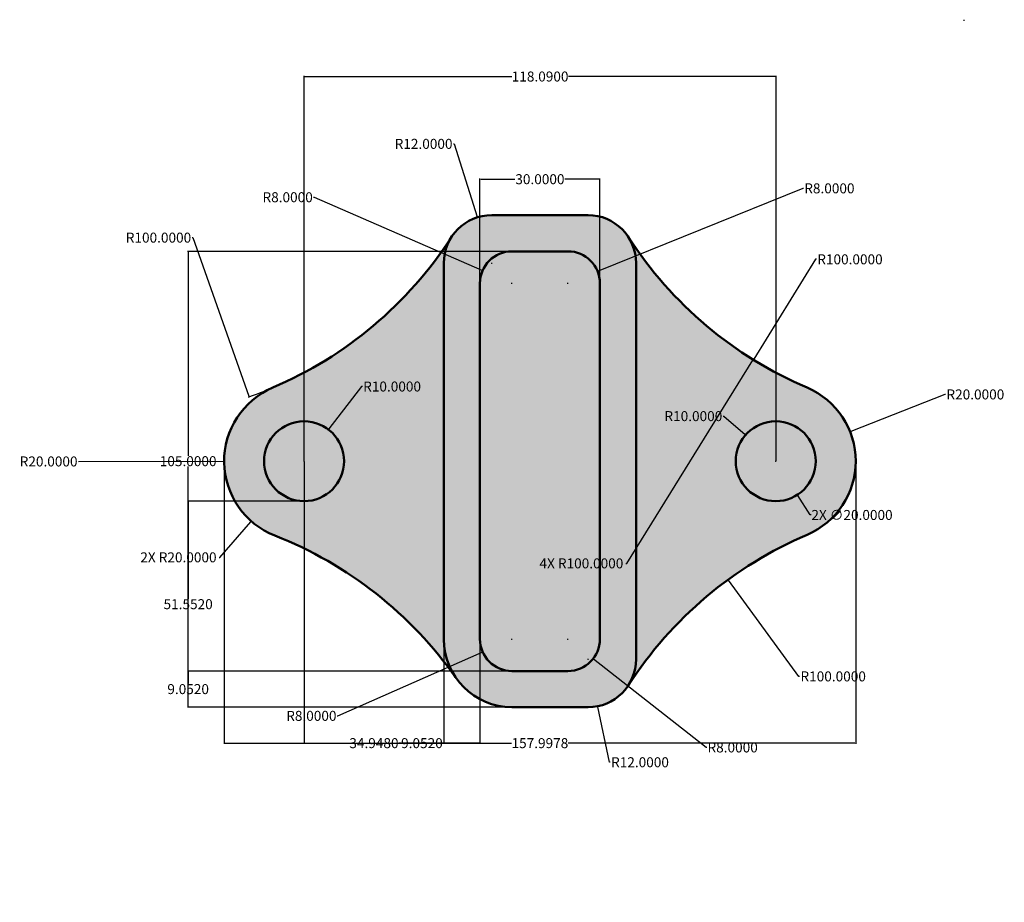
# Model space of a CAD drawing. Units: inches. Extents: x 2167893 to 2168140, y 2398931 to 2399152.
import ezdxf

# ---------------------------------------------------------------- set-up
doc = ezdxf.new("R2010")
doc.units = ezdxf.units.IN
doc.header["$MEASUREMENT"] = 0
for name, color, linetype, lineweight in [('M-DIMS', 2, 'Continuous', 25), ('M-HATC', 8, 'Continuous', 18), ('M-OUTL', 7, 'Continuous', 50)]:
    doc.layers.add(name, color=color, linetype=linetype, lineweight=lineweight)
doc.styles.get("Standard").update_dxf_attribs({"font": 'arial.ttf'})
doc.dimstyles.get("Standard").update_dxf_attribs({"dimtxt": 2.5, "dimasz": 0.18, "dimexe": 0.18, "dimexo": 0.0625, "dimgap": 0.09, "dimtad": 0, "dimtih": 1, "dimtoh": 1, "dimdec": 4, "dimzin": 0, "dimdsep": 46, "dimtxsty": 'Standard', "dimcen": 0.09, "dimadec": 0, "dimazin": 0, "dimtfac": 1, "dimtdec": 4, "dimtofl": 0, "dimtmove": 0, "dimatfit": 3, "dimfxl": 1, "dimtolj": 1, "dimtzin": 0, "dimarcsym": 0})

# ---------------------------------------------------------------- blocks, each defined once
blk = doc.blocks.new('*D1')
at = {"layer": 'Defpoints', "color": 0, "transparency": 16777216}
for p in [(2168070.68, 2399011.55), (2168129.7, 2398930.83)]:
    blk.add_point(p, dxfattribs=at)
at = {"layer": 'M-DIMS', "color": 0, "lineweight": -2, "transparency": 16777216}
for p, q in [((2168088.38, 2398987.35), (2168070.79, 2399011.41)), ((2168088.56, 2398987.35), (2168088.38, 2398987.35))]:
    blk.add_line(p, q, dxfattribs=at)
at = {"layer": 'M-DIMS', "color": 0, "transparency": 16777216}
blk.add_solid([(2168070.81, 2399011.42), (2168070.76, 2399011.39), (2168070.68, 2399011.55)], dxfattribs=at)
at = {"layer": 'M-DIMS', "color": 0, "transparency": 16777216, "insert": (2168096.97, 2398987.35), "char_height": 2.5, "attachment_point": 5}
blk.add_mtext('\\A1;R100.0000', dxfattribs=at)
blk = doc.blocks.new('*D2')
at = {"layer": 'Defpoints', "color": 0, "transparency": 16777216}
for p in [(2168075.05, 2399047.75), (2168082.6, 2399041.2)]:
    blk.add_point(p, dxfattribs=at)
at = {"layer": 'M-DIMS', "color": 0, "lineweight": -2, "transparency": 16777216}
for p, q in [((2168069.43, 2399052.47), (2168069.61, 2399052.47)), ((2168069.61, 2399052.47), (2168074.91, 2399047.87)), ((2168082.51, 2399041.2), (2168082.69, 2399041.2)), ((2168082.6, 2399041.11), (2168082.6, 2399041.29))]:
    blk.add_line(p, q, dxfattribs=at)
at = {"layer": 'M-DIMS', "color": 0, "transparency": 16777216}
blk.add_solid([(2168074.93, 2399047.89), (2168074.9, 2399047.85), (2168075.05, 2399047.75)], dxfattribs=at)
at = {"layer": 'M-DIMS', "color": 0, "transparency": 16777216, "insert": (2168061.99, 2399052.47), "char_height": 2.5, "attachment_point": 5}
blk.add_mtext('\\A1;R10.0000', dxfattribs=at)
blk = doc.blocks.new('*D3')
at = {"layer": 'Defpoints', "color": 0, "transparency": 16777216}
for p in [(2168101.21, 2399048.54), (2168082.6, 2399041.2)]:
    blk.add_point(p, dxfattribs=at)
at = {"layer": 'M-DIMS', "color": 0, "lineweight": -2, "transparency": 16777216}
for p, q in [((2168124.92, 2399057.9), (2168101.37, 2399048.61)), ((2168125.1, 2399057.9), (2168124.92, 2399057.9)), ((2168082.51, 2399041.2), (2168082.69, 2399041.2)), ((2168082.6, 2399041.11), (2168082.6, 2399041.29))]:
    blk.add_line(p, q, dxfattribs=at)
at = {"layer": 'M-DIMS', "color": 0, "transparency": 16777216}
blk.add_solid([(2168101.36, 2399048.63), (2168101.38, 2399048.58), (2168101.21, 2399048.54)], dxfattribs=at)
at = {"layer": 'M-DIMS', "color": 0, "transparency": 16777216, "insert": (2168132.54, 2399057.9), "char_height": 2.5, "attachment_point": 5}
blk.add_mtext('\\A1;R20.0000', dxfattribs=at)
blk = doc.blocks.new('*D4')
at = {"layer": 'Defpoints', "color": 0, "transparency": 16777216}
for p in [(2168129.7, 2399151.57), (2168077, 2399066.58)]:
    blk.add_point(p, dxfattribs=at)
at = {"layer": 'M-DIMS', "color": 0, "lineweight": -2, "transparency": 16777216}
for p, q in [((2168092.58, 2399091.7), (2168077.1, 2399066.74)), ((2168092.76, 2399091.7), (2168092.58, 2399091.7))]:
    blk.add_line(p, q, dxfattribs=at)
at = {"layer": 'M-DIMS', "color": 0, "transparency": 16777216}
blk.add_solid([(2168077.07, 2399066.75), (2168077.12, 2399066.72), (2168077, 2399066.58)], dxfattribs=at)
at = {"layer": 'M-DIMS', "color": 0, "transparency": 16777216, "insert": (2168101.17, 2399091.7), "char_height": 2.5, "attachment_point": 5}
blk.add_mtext('\\A1;R100.0000', dxfattribs=at)
blk = doc.blocks.new('*D5')
at = {"layer": 'Defpoints', "color": 0, "transparency": 16777216}
for p in [(2168030.6, 2398996.7), (2168036.9, 2398991.76)]:
    blk.add_point(p, dxfattribs=at)
at = {"layer": 'M-DIMS', "color": 0, "lineweight": -2, "transparency": 16777216}
for p, q in [((2168030.51, 2398996.7), (2168030.69, 2398996.7)), ((2168030.6, 2398996.61), (2168030.6, 2398996.79)), ((2168065.17, 2398969.58), (2168037.04, 2398991.65)), ((2168065.35, 2398969.58), (2168065.17, 2398969.58))]:
    blk.add_line(p, q, dxfattribs=at)
at = {"layer": 'M-DIMS', "color": 0, "transparency": 16777216}
blk.add_solid([(2168037.06, 2398991.67), (2168037.02, 2398991.63), (2168036.9, 2398991.76)], dxfattribs=at)
at = {"layer": 'M-DIMS', "color": 0, "transparency": 16777216, "insert": (2168071.82, 2398969.58), "char_height": 2.5, "attachment_point": 5}
blk.add_mtext('\\A1;R8.0000', dxfattribs=at)
blk = doc.blocks.new('*D6')
at = {"layer": 'Defpoints', "color": 0, "transparency": 16777216}
for p in [(2168016.6, 2398996.7), (2168009.28, 2398993.47)]:
    blk.add_point(p, dxfattribs=at)
at = {"layer": 'M-DIMS', "color": 0, "lineweight": -2, "transparency": 16777216}
for p, q in [((2168016.51, 2398996.7), (2168016.69, 2398996.7)), ((2168016.6, 2398996.61), (2168016.6, 2398996.79)), ((2167973.07, 2398977.48), (2168009.12, 2398993.39)), ((2167972.89, 2398977.48), (2167973.07, 2398977.48))]:
    blk.add_line(p, q, dxfattribs=at)
at = {"layer": 'M-DIMS', "color": 0, "transparency": 16777216}
blk.add_solid([(2168009.11, 2398993.42), (2168009.13, 2398993.37), (2168009.28, 2398993.47)], dxfattribs=at)
at = {"layer": 'M-DIMS', "color": 0, "transparency": 16777216, "insert": (2167966.42, 2398977.48), "char_height": 2.5, "attachment_point": 5}
blk.add_mtext('\\A1;R8.0000', dxfattribs=at)
blk = doc.blocks.new('*D7')
at = {"layer": 'Defpoints', "color": 0, "transparency": 16777216}
for p in [(2168038.02, 2399088.7), (2168030.6, 2399085.7)]:
    blk.add_point(p, dxfattribs=at)
at = {"layer": 'M-DIMS', "color": 0, "lineweight": -2, "transparency": 16777216}
for p, q in [((2168089.37, 2399109.46), (2168038.19, 2399088.76)), ((2168089.55, 2399109.46), (2168089.37, 2399109.46)), ((2168030.51, 2399085.7), (2168030.69, 2399085.7)), ((2168030.6, 2399085.61), (2168030.6, 2399085.79))]:
    blk.add_line(p, q, dxfattribs=at)
at = {"layer": 'M-DIMS', "color": 0, "transparency": 16777216}
blk.add_solid([(2168038.17, 2399088.79), (2168038.2, 2399088.74), (2168038.02, 2399088.7)], dxfattribs=at)
at = {"layer": 'M-DIMS', "color": 0, "transparency": 16777216, "insert": (2168096.02, 2399109.46), "char_height": 2.5, "attachment_point": 5}
blk.add_mtext('\\A1;R8.0000', dxfattribs=at)
blk = doc.blocks.new('*D8')
at = {"layer": 'Defpoints', "color": 0, "transparency": 16777216}
for p in [(2168009.27, 2399088.89), (2168016.6, 2399085.7)]:
    blk.add_point(p, dxfattribs=at)
at = {"layer": 'M-DIMS', "color": 0, "lineweight": -2, "transparency": 16777216}
for p, q in [((2167966.97, 2399107.24), (2167967.15, 2399107.24)), ((2167967.15, 2399107.24), (2168009.1, 2399088.96)), ((2168016.51, 2399085.7), (2168016.69, 2399085.7)), ((2168016.6, 2399085.61), (2168016.6, 2399085.79))]:
    blk.add_line(p, q, dxfattribs=at)
at = {"layer": 'M-DIMS', "color": 0, "transparency": 16777216}
blk.add_solid([(2168009.11, 2399088.99), (2168009.09, 2399088.94), (2168009.27, 2399088.89)], dxfattribs=at)
at = {"layer": 'M-DIMS', "color": 0, "transparency": 16777216, "insert": (2167960.49, 2399107.24), "char_height": 2.5, "attachment_point": 5}
blk.add_mtext('\\A1;R8.0000', dxfattribs=at)
blk = doc.blocks.new('*D9')
at = {"layer": 'Defpoints', "color": 0, "transparency": 16777216}
for p in [(2167917.5, 2399151.57), (2167950.88, 2399057.3)]:
    blk.add_point(p, dxfattribs=at)
at = {"layer": 'M-DIMS', "color": 0, "lineweight": -2, "transparency": 16777216}
for p, q in [((2167936.6, 2399097.13), (2167936.78, 2399097.13)), ((2167936.78, 2399097.13), (2167950.82, 2399057.47))]:
    blk.add_line(p, q, dxfattribs=at)
blk.add_arc((2167917.5, 2399151.57), 100, 289.3936, 293.0748, dxfattribs=at)
at = {"layer": 'M-DIMS', "color": 0, "transparency": 16777216}
blk.add_solid([(2167950.84, 2399057.48), (2167950.79, 2399057.46), (2167950.88, 2399057.3)], dxfattribs=at)
at = {"layer": 'M-DIMS', "color": 0, "transparency": 16777216, "insert": (2167928.18, 2399097.13), "char_height": 2.5, "attachment_point": 5}
blk.add_mtext('\\A1;R100.0000', dxfattribs=at)
blk = doc.blocks.new('*D10')
at = {"layer": 'Defpoints', "color": 0, "transparency": 16777216}
for p in [(2167970.71, 2399049.12), (2167964.6, 2399041.2)]:
    blk.add_point(p, dxfattribs=at)
at = {"layer": 'M-DIMS', "color": 0, "lineweight": -2, "transparency": 16777216}
for p, q in [((2167979, 2399059.88), (2167970.82, 2399049.26)), ((2167979.18, 2399059.88), (2167979, 2399059.88)), ((2167964.51, 2399041.2), (2167964.69, 2399041.2)), ((2167964.6, 2399041.11), (2167964.6, 2399041.29))]:
    blk.add_line(p, q, dxfattribs=at)
at = {"layer": 'M-DIMS', "color": 0, "transparency": 16777216}
blk.add_solid([(2167970.79, 2399049.28), (2167970.84, 2399049.24), (2167970.71, 2399049.12)], dxfattribs=at)
at = {"layer": 'M-DIMS', "color": 0, "transparency": 16777216, "insert": (2167986.62, 2399059.88), "char_height": 2.5, "attachment_point": 5}
blk.add_mtext('\\A1;R10.0000', dxfattribs=at)
blk = doc.blocks.new('*D11')
at = {"layer": 'Defpoints', "color": 0, "transparency": 16777216}
for p in [(2167944.6, 2399041.17), (2167964.6, 2399041.2)]:
    blk.add_point(p, dxfattribs=at)
at = {"layer": 'M-DIMS', "color": 0, "lineweight": -2, "transparency": 16777216}
for p, q in [((2167908.13, 2399041.13), (2167944.42, 2399041.17)), ((2167964.51, 2399041.2), (2167964.69, 2399041.2)), ((2167964.6, 2399041.11), (2167964.6, 2399041.29))]:
    blk.add_line(p, q, dxfattribs=at)
at = {"layer": 'M-DIMS', "color": 0, "transparency": 16777216}
blk.add_solid([(2167944.42, 2399041.2), (2167944.42, 2399041.14), (2167944.6, 2399041.17)], dxfattribs=at)
at = {"layer": 'M-DIMS', "color": 0, "transparency": 16777216, "insert": (2167900.69, 2399041.13), "char_height": 2.5, "attachment_point": 5}
blk.add_mtext('\\A1;R20.0000', dxfattribs=at)
blk = doc.blocks.new('*D12')
at = {"layer": 'Defpoints', "color": 0, "transparency": 16777216}
for p in [(2168007.94, 2399102.19), (2168011.55, 2399090.75)]:
    blk.add_point(p, dxfattribs=at)
at = {"layer": 'M-DIMS', "color": 0, "lineweight": -2, "transparency": 16777216}
for p, q in [((2168001.95, 2399120.59), (2168002.13, 2399120.59)), ((2168002.13, 2399120.59), (2168007.88, 2399102.36)), ((2168011.46, 2399090.75), (2168011.64, 2399090.75)), ((2168011.55, 2399090.66), (2168011.55, 2399090.84))]:
    blk.add_line(p, q, dxfattribs=at)
at = {"layer": 'M-DIMS', "color": 0, "transparency": 16777216}
blk.add_solid([(2168007.91, 2399102.37), (2168007.85, 2399102.36), (2168007.94, 2399102.19)], dxfattribs=at)
at = {"layer": 'M-DIMS', "color": 0, "transparency": 16777216, "insert": (2167994.5, 2399120.59), "char_height": 2.5, "attachment_point": 5}
blk.add_mtext('\\A1;R12.0000', dxfattribs=at)
blk = doc.blocks.new('*D13')
at = {"layer": 'Defpoints', "color": 0, "transparency": 16777216}
for p in [(2168035.65, 2398991.65), (2168038.1, 2398979.9)]:
    blk.add_point(p, dxfattribs=at)
at = {"layer": 'M-DIMS', "color": 0, "lineweight": -2, "transparency": 16777216}
for p, q in [((2168035.56, 2398991.65), (2168035.74, 2398991.65)), ((2168035.65, 2398991.56), (2168035.65, 2398991.74)), ((2168041.01, 2398965.87), (2168038.13, 2398979.72)), ((2168041.19, 2398965.87), (2168041.01, 2398965.87))]:
    blk.add_line(p, q, dxfattribs=at)
at = {"layer": 'M-DIMS', "color": 0, "transparency": 16777216}
blk.add_solid([(2168038.16, 2398979.73), (2168038.1, 2398979.71), (2168038.1, 2398979.9)], dxfattribs=at)
at = {"layer": 'M-DIMS', "color": 0, "transparency": 16777216, "insert": (2168048.64, 2398965.87), "char_height": 2.5, "attachment_point": 5}
blk.add_mtext('\\A1;R12.0000', dxfattribs=at)
blk = doc.blocks.new('*D14')
at = {"layer": 'Defpoints', "color": 0, "transparency": 16777216}
for p in [(2167964.6, 2399137.44), (2167964.6, 2399041.29), (2168082.69, 2399041.2)]:
    blk.add_point(p, dxfattribs=at)
at = {"layer": 'M-DIMS', "color": 0, "lineweight": -2, "transparency": 16777216}
for p, q in [((2167964.6, 2399041.35), (2167964.6, 2399137.62)), ((2167964.78, 2399137.44), (2168016.55, 2399137.44)), ((2168082.51, 2399137.44), (2168030.75, 2399137.44)), ((2168082.69, 2399041.26), (2168082.69, 2399137.62))]:
    blk.add_line(p, q, dxfattribs=at)
at = {"layer": 'M-DIMS', "color": 0, "transparency": 16777216}
for points in [[(2167964.78, 2399137.47), (2167964.78, 2399137.41), (2167964.6, 2399137.44)], [(2168082.51, 2399137.47), (2168082.51, 2399137.41), (2168082.69, 2399137.44)]]:
    blk.add_solid(points, dxfattribs=at)
at = {"layer": 'M-DIMS', "color": 0, "transparency": 16777216, "insert": (2168023.65, 2399137.44), "char_height": 2.5, "attachment_point": 5}
blk.add_mtext('\\A1;118.0900', dxfattribs=at)
blk = doc.blocks.new('*D15')
at = {"layer": 'Defpoints', "color": 0, "transparency": 16777216}
for p in [(2168102.6, 2399041.2), (2167944.6, 2399040.9), (2168102.6, 2398970.65)]:
    blk.add_point(p, dxfattribs=at)
at = {"layer": 'M-DIMS', "color": 0, "lineweight": -2, "transparency": 16777216}
for p, q in [((2167944.6, 2399040.84), (2167944.6, 2398970.47)), ((2168102.6, 2399041.14), (2168102.6, 2398970.47)), ((2167944.78, 2398970.65), (2168016.5, 2398970.65)), ((2168102.42, 2398970.65), (2168030.71, 2398970.65))]:
    blk.add_line(p, q, dxfattribs=at)
at = {"layer": 'M-DIMS', "color": 0, "transparency": 16777216}
for points in [[(2167944.78, 2398970.68), (2167944.78, 2398970.62), (2167944.6, 2398970.65)], [(2168102.42, 2398970.68), (2168102.42, 2398970.62), (2168102.6, 2398970.65)]]:
    blk.add_solid(points, dxfattribs=at)
at = {"layer": 'M-DIMS', "color": 0, "transparency": 16777216, "insert": (2168023.6, 2398970.65), "char_height": 2.5, "attachment_point": 5}
blk.add_mtext('\\A1;157.9978', dxfattribs=at)
blk = doc.blocks.new('*D16')
at = {"layer": 'Defpoints', "color": 0, "transparency": 16777216}
for p in [(2168038.6, 2399111.75), (2168008.6, 2399085.7), (2168038.6, 2399085.7)]:
    blk.add_point(p, dxfattribs=at)
at = {"layer": 'M-DIMS', "color": 0, "lineweight": -2, "transparency": 16777216}
for p, q in [((2168008.6, 2399085.76), (2168008.6, 2399111.93)), ((2168008.78, 2399111.75), (2168017.36, 2399111.75)), ((2168038.42, 2399111.75), (2168029.85, 2399111.75)), ((2168038.6, 2399085.76), (2168038.6, 2399111.93))]:
    blk.add_line(p, q, dxfattribs=at)
at = {"layer": 'M-DIMS', "color": 0, "transparency": 16777216}
for points in [[(2168008.78, 2399111.78), (2168008.78, 2399111.72), (2168008.6, 2399111.75)], [(2168038.42, 2399111.78), (2168038.42, 2399111.72), (2168038.6, 2399111.75)]]:
    blk.add_solid(points, dxfattribs=at)
at = {"layer": 'M-DIMS', "color": 0, "transparency": 16777216, "insert": (2168023.6, 2399111.75), "char_height": 2.5, "attachment_point": 5}
blk.add_mtext('\\A1;30.0000', dxfattribs=at)
blk = doc.blocks.new('*D17')
at = {"layer": 'Defpoints', "color": 0, "transparency": 16777216}
for p in [(2168016.6, 2399093.7), (2167935.6, 2398988.7), (2168016.6, 2398988.7)]:
    blk.add_point(p, dxfattribs=at)
at = {"layer": 'M-DIMS', "color": 0, "lineweight": -2, "transparency": 16777216}
for p, q in [((2168016.54, 2399093.7), (2167935.42, 2399093.7)), ((2167935.6, 2399093.52), (2167935.6, 2399042.56)), ((2167935.6, 2398988.88), (2167935.6, 2399039.83)), ((2168016.54, 2398988.7), (2167935.42, 2398988.7))]:
    blk.add_line(p, q, dxfattribs=at)
at = {"layer": 'M-DIMS', "color": 0, "transparency": 16777216}
for points in [[(2167935.57, 2399093.52), (2167935.63, 2399093.52), (2167935.6, 2399093.7)], [(2167935.57, 2398988.88), (2167935.63, 2398988.88), (2167935.6, 2398988.7)]]:
    blk.add_solid(points, dxfattribs=at)
at = {"layer": 'M-DIMS', "color": 0, "transparency": 16777216, "insert": (2167935.6, 2399041.2), "char_height": 2.5, "attachment_point": 5}
blk.add_mtext('\\A1;105.0000', dxfattribs=at)
blk = doc.blocks.new('*D18')
at = {"layer": 'Defpoints', "color": 0, "transparency": 16777216}
for p in [(2167964.6, 2399041.2), (2167999.55, 2398996.7), (2167999.55, 2398970.65)]:
    blk.add_point(p, dxfattribs=at)
at = {"layer": 'M-DIMS', "color": 0, "lineweight": -2, "transparency": 16777216}
for p, q in [((2167964.6, 2399041.14), (2167964.6, 2398970.47)), ((2167999.55, 2398996.64), (2167999.55, 2398970.47)), ((2167964.78, 2398970.65), (2167975.83, 2398970.65)), ((2167999.37, 2398970.65), (2167988.32, 2398970.65))]:
    blk.add_line(p, q, dxfattribs=at)
at = {"layer": 'M-DIMS', "color": 0, "transparency": 16777216}
for points in [[(2167964.78, 2398970.68), (2167964.78, 2398970.62), (2167964.6, 2398970.65)], [(2167999.37, 2398970.68), (2167999.37, 2398970.62), (2167999.55, 2398970.65)]]:
    blk.add_solid(points, dxfattribs=at)
at = {"layer": 'M-DIMS', "color": 0, "transparency": 16777216, "insert": (2167982.08, 2398970.65), "char_height": 2.5, "attachment_point": 5}
blk.add_mtext('\\A1;34.9480', dxfattribs=at)
blk = doc.blocks.new('*D19')
at = {"layer": 'Defpoints', "color": 0, "transparency": 16777216}
for p in [(2167964.6, 2399031.2), (2167935.6, 2398979.65), (2168016.6, 2398979.65)]:
    blk.add_point(p, dxfattribs=at)
at = {"layer": 'M-DIMS', "color": 0, "lineweight": -2, "transparency": 16777216}
for p, q in [((2167964.54, 2399031.2), (2167935.42, 2399031.2)), ((2167935.6, 2399031.02), (2167935.6, 2399006.79)), ((2167935.6, 2398979.83), (2167935.6, 2399004.06)), ((2168016.54, 2398979.65), (2167935.42, 2398979.65))]:
    blk.add_line(p, q, dxfattribs=at)
at = {"layer": 'M-DIMS', "color": 0, "transparency": 16777216}
for points in [[(2167935.57, 2399031.02), (2167935.63, 2399031.02), (2167935.6, 2399031.2)], [(2167935.57, 2398979.83), (2167935.63, 2398979.83), (2167935.6, 2398979.65)]]:
    blk.add_solid(points, dxfattribs=at)
at = {"layer": 'M-DIMS', "color": 0, "transparency": 16777216, "insert": (2167935.6, 2399005.42), "char_height": 2.5, "attachment_point": 5}
blk.add_mtext('\\A1;51.5520', dxfattribs=at)
blk = doc.blocks.new('*D20')
at = {"layer": 'Defpoints', "color": 0, "transparency": 16777216}
for p in [(2167999.55, 2398996.7), (2168008.6, 2398996.7), (2167999.55, 2398970.65)]:
    blk.add_point(p, dxfattribs=at)
at = {"layer": 'M-DIMS', "color": 0, "lineweight": -2, "transparency": 16777216}
for p, q in [((2167999.55, 2398996.64), (2167999.55, 2398970.47)), ((2168008.6, 2398996.64), (2168008.6, 2398970.47)), ((2167999.55, 2398970.65), (2167999.37, 2398970.65)), ((2168008.42, 2398970.65), (2167999.73, 2398970.65))]:
    blk.add_line(p, q, dxfattribs=at)
at = {"layer": 'M-DIMS', "color": 0, "transparency": 16777216}
for points in [[(2167999.73, 2398970.68), (2167999.73, 2398970.62), (2167999.55, 2398970.65)], [(2168008.42, 2398970.68), (2168008.42, 2398970.62), (2168008.6, 2398970.65)]]:
    blk.add_solid(points, dxfattribs=at)
at = {"layer": 'M-DIMS', "color": 0, "transparency": 16777216, "insert": (2167994.09, 2398970.65), "char_height": 2.5, "attachment_point": 5}
blk.add_mtext('\\A1;9.0520', dxfattribs=at)
blk = doc.blocks.new('*D21')
at = {"layer": 'Defpoints', "color": 0, "transparency": 16777216}
for p in [(2167935.6, 2398988.7), (2168016.6, 2398988.7), (2168016.6, 2398979.65)]:
    blk.add_point(p, dxfattribs=at)
at = {"layer": 'M-DIMS', "color": 0, "lineweight": -2, "transparency": 16777216}
for p, q in [((2168016.54, 2398988.7), (2167935.42, 2398988.7)), ((2167935.6, 2398988.52), (2167935.6, 2398985.54)), ((2167935.6, 2398979.83), (2167935.6, 2398982.81)), ((2168016.54, 2398979.65), (2167935.42, 2398979.65))]:
    blk.add_line(p, q, dxfattribs=at)
at = {"layer": 'M-DIMS', "color": 0, "transparency": 16777216}
for points in [[(2167935.57, 2398988.52), (2167935.63, 2398988.52), (2167935.6, 2398988.7)], [(2167935.57, 2398979.83), (2167935.63, 2398979.83), (2167935.6, 2398979.65)]]:
    blk.add_solid(points, dxfattribs=at)
at = {"layer": 'M-DIMS', "color": 0, "transparency": 16777216, "insert": (2167935.6, 2398984.17), "char_height": 2.5, "attachment_point": 5}
blk.add_mtext('\\A1;9.0520', dxfattribs=at)
blk = doc.blocks.new('*D22')
at = {"layer": 'Defpoints', "color": 0, "transparency": 16777216}
for p in [(2167964.6, 2399041.2), (2167951.41, 2399026.16)]:
    blk.add_point(p, dxfattribs=at)
at = {"layer": 'M-DIMS', "color": 0, "lineweight": -2, "transparency": 16777216}
for p, q in [((2167964.51, 2399041.2), (2167964.69, 2399041.2)), ((2167964.6, 2399041.11), (2167964.6, 2399041.29)), ((2167943.5, 2399017.14), (2167951.29, 2399026.03)), ((2167943.32, 2399017.14), (2167943.5, 2399017.14))]:
    blk.add_line(p, q, dxfattribs=at)
at = {"layer": 'M-DIMS', "color": 0, "transparency": 16777216}
blk.add_solid([(2167951.27, 2399026.05), (2167951.32, 2399026.01), (2167951.41, 2399026.16)], dxfattribs=at)
at = {"layer": 'M-DIMS', "color": 0, "transparency": 16777216, "insert": (2167933.17, 2399017.14), "char_height": 2.5, "attachment_point": 5}
blk.add_mtext('\\A1;2X R20.0000', dxfattribs=at)
blk = doc.blocks.new('*D23')
at = {"layer": 'Defpoints', "color": 0, "transparency": 16777216}
for p in [(2168077.19, 2399049.61), (2168088.01, 2399032.79)]:
    blk.add_point(p, dxfattribs=at)
at = {"layer": 'M-DIMS', "color": 0, "lineweight": -2, "transparency": 16777216}
for p, q in [((2168082.51, 2399041.2), (2168082.69, 2399041.2)), ((2168082.6, 2399041.11), (2168082.6, 2399041.29)), ((2168091.25, 2399027.74), (2168088.11, 2399032.63)), ((2168091.43, 2399027.74), (2168091.25, 2399027.74))]:
    blk.add_line(p, q, dxfattribs=at)
at = {"layer": 'M-DIMS', "color": 0, "transparency": 16777216}
blk.add_solid([(2168088.13, 2399032.65), (2168088.08, 2399032.62), (2168088.01, 2399032.79)], dxfattribs=at)
at = {"layer": 'M-DIMS', "color": 0, "transparency": 16777216, "insert": (2168101.68, 2399027.74), "char_height": 2.5, "attachment_point": 5}
blk.add_mtext('\\A1;2X ∅20.0000', dxfattribs=at)
blk = doc.blocks.new('*D24')
at = {"layer": 'Defpoints', "color": 0, "transparency": 16777216}
for p in [(2168129.7, 2399151.57), (2168076.96, 2399066.61)]:
    blk.add_point(p, dxfattribs=at)
at = {"layer": 'M-DIMS', "color": 0, "lineweight": -2, "transparency": 16777216}
for p, q in [((2168129.61, 2399151.57), (2168129.79, 2399151.57)), ((2168129.7, 2399151.48), (2168129.7, 2399151.66)), ((2168045.31, 2399015.63), (2168076.86, 2399066.46)), ((2168045.13, 2399015.63), (2168045.31, 2399015.63))]:
    blk.add_line(p, q, dxfattribs=at)
at = {"layer": 'M-DIMS', "color": 0, "transparency": 16777216}
blk.add_solid([(2168076.84, 2399066.47), (2168076.89, 2399066.44), (2168076.96, 2399066.61)], dxfattribs=at)
at = {"layer": 'M-DIMS', "color": 0, "transparency": 16777216, "insert": (2168033.98, 2399015.63), "char_height": 2.5, "attachment_point": 5}
blk.add_mtext('\\A1;4X R100.0000', dxfattribs=at)

msp = doc.modelspace()

# ---------------------------------------------------------------- hatches: boundary and pattern name
at = {"layer": 'M-HATC'}
h = msp.add_hatch(color=256, dxfattribs=at)
h.dxf.hatch_style = 1
h.paths.add_polyline_path([(2168035.65379, 2399102.74978), (2168011.54983, 2399102.74978, 0.414213562), (2167999.54983, 2399090.74978), (2167999.54983, 2398996.6978, 0.414213562), (2168016.60181, 2398979.64582), (2168035.65379, 2398979.64582, 0.414213562), (2168047.65379, 2398991.64582), (2168047.65379, 2399090.74978, 0.414213562)])
h.paths.add_polyline_path([(2168038.60181, 2399085.6978), (2168038.60181, 2398996.6978, -0.414213562), (2168030.60181, 2398988.6978), (2168016.60181, 2398988.6978, -0.414213562), (2168008.60181, 2398996.6978), (2168008.60181, 2399085.6978, -0.414213562), (2168016.60181, 2399093.6978), (2168030.60181, 2399093.6978, -0.414213562)], flags=16)
h = msp.add_hatch(color=256, dxfattribs=at)
h.dxf.hatch_style = 1
h.paths.add_polyline_path([(2168045.73049, 2399097.26593, -0.144498329), (2168047.65379, 2399090.74978), (2168047.65379, 2398991.64582, -0.144499795), (2168045.73045, 2398985.12962, -0.149451771), (2168090.45194, 2399022.80282, 0.660498894), (2168090.45194, 2399059.59279, -0.149451595)])
h.paths.add_polyline_path([(2168092.60181, 2399041.1978, -1), (2168072.60181, 2399041.1978, -1)], flags=16)
h.paths.add_polyline_path([(2167999.54983, 2399090.74978, -0.144499795), (2168001.47317, 2399097.26599, -0.149451771), (2167956.75167, 2399059.59279, 0.671110123), (2167957.29596, 2399022.57995, -0.147369541), (2168002.64067, 2398986.90715, -0.154098603), (2167999.54983, 2398996.6978)])
h.paths.add_polyline_path([(2167974.60181, 2399041.1978, -1), (2167954.60181, 2399041.1978, -1)], flags=16)
h.paths.add_polyline_path([(2168053.73949, 2399049.88046), (2168070.13615, 2399049.88046), (2168070.13615, 2399055.03223), (2168053.73949, 2399055.03223)], flags=24)
h.paths.add_polyline_path([(2167978.36829, 2399057.28141), (2167994.76495, 2399057.28141), (2167994.76495, 2399062.43318), (2167978.36829, 2399062.43318)], flags=24)
h = msp.add_hatch(color=256, dxfattribs=at)
h.dxf.hatch_style = 1
h.set_gradient(color1=(19, 103, 52), color2=(255, 255, 0))
h.paths.add_polyline_path([(2168038.60181, 2399085.6978, 0.414213562), (2168030.60181, 2399093.6978), (2168016.60181, 2399093.6978, 0.414213562), (2168008.60181, 2399085.6978), (2168008.60181, 2398996.6978, 0.414213562), (2168016.60181, 2398988.6978), (2168030.60181, 2398988.6978, 0.414213562), (2168038.60181, 2398996.6978)])
h = msp.add_hatch(color=256, dxfattribs=at)
h.dxf.hatch_style = 1
h.paths.add_polyline_path([(2167954.60181, 2399041.1978, 1), (2167974.60181, 2399041.1978, 1)])
h.paths.add_polyline_path([(2168072.60181, 2399041.1978, 1), (2168092.60181, 2399041.1978, 1)])

# ---------------------------------------------------------------- linework, layer by layer
at = {"layer": 'M-OUTL'}
for points in [[(2168016.60181, 2398979.64582), (2168035.65379, 2398979.64582, 0.414213562), (2168047.65379, 2398991.64582), (2168047.65379, 2399090.74978, 0.414213562), (2168035.65379, 2399102.74978), (2168011.54983, 2399102.74978, 0.414213562), (2167999.54983, 2399090.74978), (2167999.54983, 2398996.6978, 0.414213562)], [(2168016.60181, 2398988.6978), (2168030.60181, 2398988.6978, 0.414213562), (2168038.60181, 2398996.6978), (2168038.60181, 2399085.6978, 0.414213562), (2168030.60181, 2399093.6978), (2168016.60181, 2399093.6978, 0.414213562), (2168008.60181, 2399085.6978), (2168008.60181, 2398996.6978, 0.414213562)]]:
    msp.add_lwpolyline(points, format="xyb", close=True, dxfattribs=at)
for centre in [(2167964.60181, 2399041.1978), (2168082.60181, 2399041.1978)]:
    msp.add_circle(centre, 10, dxfattribs=at)
for centre, radius, start, end in [((2167917.501, 2399151.5677), 100, 293.1105644, 327.1107369), ((2168129.70261, 2399151.5677), 100, 212.8892631, 246.8894356), ((2167964.60181, 2399041.1978), 20, 113.1105644, 248.5744114), ((2168082.60181, 2399041.1978), 20, 293.1105644, 66.8894356), ((2167920.7667, 2398929.49067), 100, 35.0411662, 68.5744114), ((2168129.70261, 2398930.82791), 100, 113.1105644, 147.1107369)]:
    msp.add_arc(centre, radius, start, end, dxfattribs=at)

# ---------------------------------------------------------------- dimensions: what is measured, and where the dimension line sits
at = {"layer": 'M-DIMS'}
for center, mpoint, picture, middle in [((2167917.501, 2399151.5677), (2167950.87639, 2399057.30167), '*D9', (2167928.18247, 2399097.12665)), ((2168129.70261, 2399151.5677), (2168077.00097, 2399066.58219), '*D4', (2168101.17038, 2399091.69929)), ((2168011.54983, 2399090.74978), (2168007.93616, 2399102.19275), '*D12', (2167994.50356, 2399120.59095)), ((2168030.60181, 2399085.6978), (2168038.01835, 2399088.69695), '*D7', (2168096.01818, 2399109.46157)), ((2168016.60181, 2399085.6978), (2168009.26747, 2399088.89273), '*D8', (2167960.49483, 2399107.24129)), ((2167964.60181, 2399041.1978), (2167970.70659, 2399049.11813), '*D10', (2167986.62034, 2399059.8752)), ((2168082.60181, 2399041.1978), (2168101.20514, 2399048.54055), '*D3', (2168132.54448, 2399057.90161)), ((2168082.60181, 2399041.1978), (2168075.05078, 2399047.75387), '*D2', (2168061.99154, 2399052.47425)), ((2167964.60181, 2399041.1978), (2167944.60182, 2399041.17242), '*D11', (2167908.13452, 2399041.12613)), ((2168129.70261, 2398930.82791), (2168070.68068, 2399011.5522), '*D1', (2168096.9729, 2398987.34589)), ((2168016.60181, 2398996.6978), (2168009.28343, 2398993.4665), '*D6', (2167966.42069, 2398977.47795)), ((2168030.60181, 2398996.6978), (2168036.89644, 2398991.76044), '*D5', (2168071.82095, 2398969.5836)), ((2168035.65379, 2398991.64582), (2168038.09719, 2398979.89721), '*D13', (2168048.63685, 2398965.8706))]:
    dim = msp.add_radius_dim(center=center, mpoint=mpoint, dimstyle='Standard', override={"dimclrd": 0, "dimclre": 0, "dimclrt": 0}, dxfattribs=at)
    dim.commit()
    dim.dimension.update_dxf_attribs({"geometry": picture, "text_midpoint": middle, "dimtype": 164})
for center, mpoint, text, picture, middle in [((2168129.70261, 2399151.5677), (2168076.95842, 2399066.60859), '4X <>', '*D24', (2168033.98205, 2399015.63313)), ((2167964.60181, 2399041.1978), (2167951.41193, 2399026.1636), '2X <>', '*D22', (2167933.16832, 2399017.14308))]:
    dim = msp.add_radius_dim(center=center, mpoint=mpoint, text=text, dimstyle='Standard', override={"dimdec": 4, "dimlfac": 1, "dimrnd": 0, "dimzin": 0, "dimdsep": 46, "dimlunit": 2}, dxfattribs=at)
    dim.commit()
    dim.dimension.update_dxf_attribs({"geometry": picture, "text_midpoint": middle, "dimtype": 164})
for base, p1, p2, override, picture, middle in [((2167964.60181, 2399137.43791), (2168082.69181, 2399041.1978), (2167964.60181, 2399041.2878), {"dimclrd": 0, "dimclre": 0, "dimclrt": 0}, '*D14', (2168023.64681, 2399137.43791)), ((2168038.60181, 2399111.74978), (2168008.60181, 2399085.6978), (2168038.60181, 2399085.6978), {"dimdec": 4, "dimlfac": 1, "dimrnd": 0, "dimzin": 0, "dimdsep": 46, "dimlunit": 2}, '*D16', (2168023.60181, 2399111.74978)), ((2168102.60181, 2398970.64582), (2167944.60397, 2399040.90373), (2168102.60181, 2399041.1978), {"dimdec": 4, "dimlfac": 1, "dimrnd": 0, "dimzin": 0, "dimdsep": 46, "dimlunit": 2}, '*D15', (2168023.60289, 2398970.64582)), ((2167999.54983, 2398970.64582), (2167964.60181, 2399041.1978), (2167999.54983, 2398996.6978), {"dimdec": 4, "dimlfac": 1, "dimrnd": 0, "dimzin": 0, "dimdsep": 46, "dimlunit": 2}, '*D18', (2167982.07582, 2398970.64582)), ((2167999.54983, 2398970.64582), (2168008.60181, 2398996.6978), (2167999.54983, 2398996.6978), {"dimdec": 4, "dimlfac": 1, "dimrnd": 0, "dimzin": 0, "dimdsep": 46, "dimlunit": 2}, '*D20', (2167994.0948, 2398970.64582))]:
    dim = msp.add_linear_dim(base=base, p1=p1, p2=p2, dimstyle='Standard', override=override, dxfattribs=at)
    dim.commit()
    dim.dimension.update_dxf_attribs({"geometry": picture, "text_midpoint": middle})
for base, p1, p2, picture, middle in [((2167935.60397, 2398988.6978), (2168016.60181, 2399093.6978), (2168016.60181, 2398988.6978), '*D17', (2167935.60397, 2399041.1978)), ((2167935.60397, 2398979.64582), (2167964.60181, 2399031.1978), (2168016.60181, 2398979.64582), '*D19', (2167935.60397, 2399005.42181)), ((2167935.60397, 2398988.6978), (2168016.60181, 2398979.64582), (2168016.60181, 2398988.6978), '*D21', (2167935.60397, 2398984.17181))]:
    dim = msp.add_linear_dim(base=base, p1=p1, p2=p2, angle=90, dimstyle='Standard', override={"dimdec": 4, "dimlfac": 1, "dimrnd": 0, "dimzin": 0, "dimdsep": 46, "dimlunit": 2}, dxfattribs=at)
    dim.commit()
    dim.dimension.update_dxf_attribs({"geometry": picture, "text_midpoint": middle})
dim = msp.add_diameter_dim_2p(p1=(2168077.19451, 2399049.60977), p2=(2168088.0091, 2399032.78584), text='2X <>', dimstyle='Standard', override={"dimdec": 4, "dimlfac": 1, "dimrnd": 0, "dimzin": 0, "dimdsep": 46, "dimlunit": 2}, dxfattribs=at)
dim.commit()
dim.dimension.update_dxf_attribs({"geometry": '*D23', "text_midpoint": (2168101.68037, 2399027.73866), "dimtype": 163})

doc.saveas('drawing.dxf')
